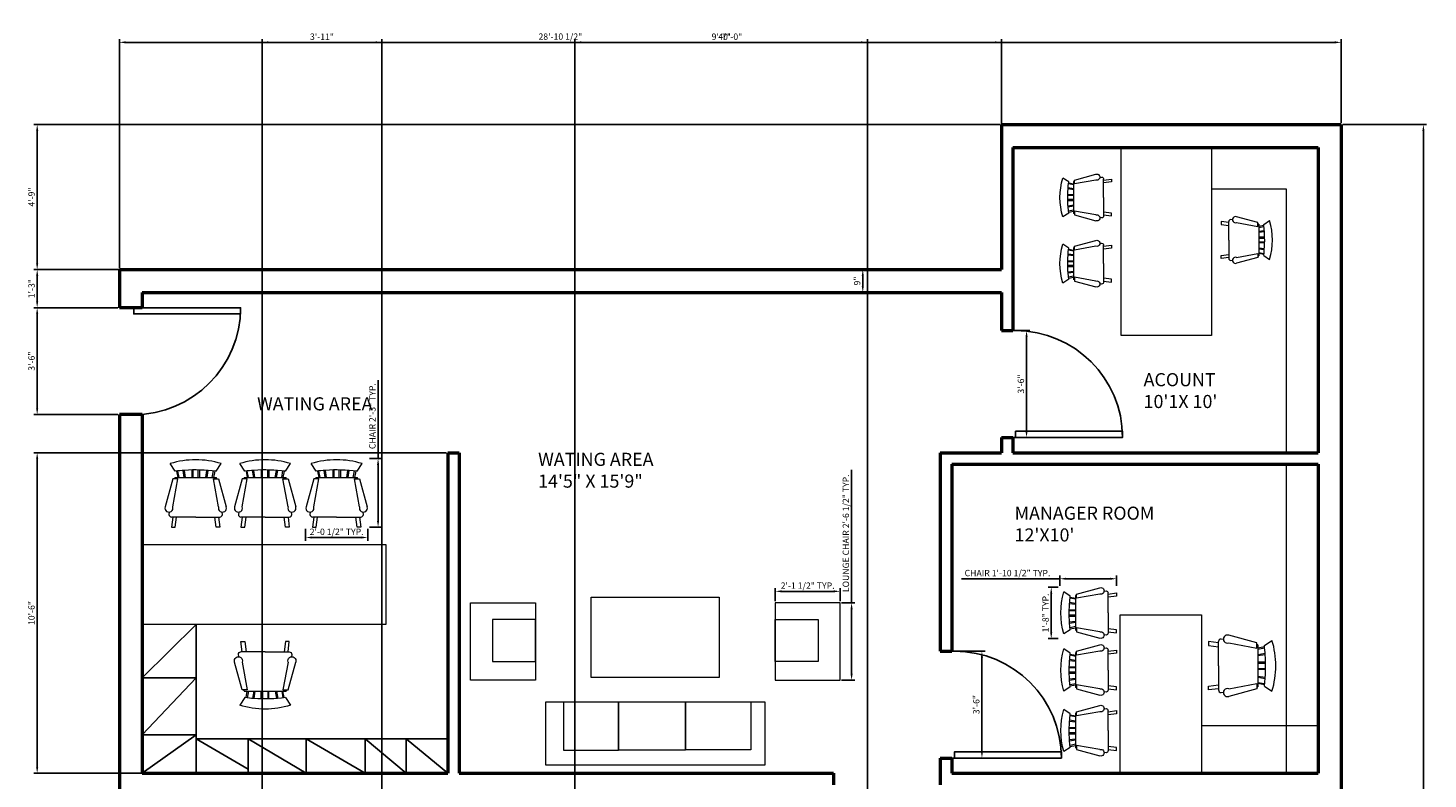
# Model space of a CAD drawing. Units: inches. Extents: x -4852 to -4300, y 4342 to 5059.
# Tile 4 of 4: x -4850 to -4300, y 4764 to 5059. Entities that reach past the tile are written whole.
import ezdxf

# ---------------------------------------------------------------- set-up
doc = ezdxf.new("R2010")
doc.units = ezdxf.units.IN
for name, color, linetype, lineweight in [('A-ANNO-DIMS', 2, 'Continuous', 18), ('A-AREA-IDEN', 7, 'Continuous', 18), ('A-DOOR', 4, 'Continuous', 25), ('A-FLOR-CASE', 9, 'Continuous', 25), ('A-FURN', 8, 'Continuous', 18), ('A-WALL', 7, 'Continuous', 50)]:
    doc.layers.add(name, color=color, linetype=linetype, lineweight=lineweight)
doc.styles.get("Standard").update_dxf_attribs({"font": 'arial.ttf'})
doc.dimstyles.new('ISO-25', dxfattribs={"dimtxt": 2.5, "dimasz": 2.5, "dimexe": 1.25, "dimexo": 0.625, "dimtad": 1, "dimdec": 0, "dimlunit": 3, "dimtxsty": 'Standard', "dimcen": 2.5, "dimadec": 0, "dimazin": 0, "dimtfac": 1, "dimtdec": 0, "dimtmove": 0, "dimatfit": 3, "dimfxl": 1, "dimarcsym": 0})

# ---------------------------------------------------------------- blocks, each defined once
blk = doc.blocks.new('*U2')
for p, q in [((0, 0), (0, -100)), ((750, 0), (750, -100))]:
    blk.add_line(p, q)
blk.add_lwpolyline([(0, 0), (0, 750), (43.75, 750), (43.75, 0)], close=True)
blk.add_arc((0, 0), 750, 0, 90)
blk = doc.blocks.new('Chair - Rocking')
for p, q in [((-8, -4.5), (-10, -1.5)), ((-7.5, -4.5), (-7, -7)), ((-6.5, -7), (-7.02225, -4.43)), ((-4.5, -7), (-4.96674, -4.19951)), ((-4, -7), (-4.40532, -4.16272)), ((-1.5, -4.05012), (-1.5, -7)), ((-1, -7), (-1, -4.05012)), ((1, -7), (1, -4.04655)), ((1.5, -4.05012), (1.5, -7)), ((4, -7), (4.40187, -4.18694)), ((4.5, -7), (4.96761, -4.19437)), ((6.5, -7), (7, -4.4057)), ((7.5, -4.5), (7, -7)), ((8, -4.5), (10, -1.5)), ((-9, -7.5), (-12, -18.49999)), ((-7, -7.5), (-9, -7.5)), ((-9, -18.49999), (-7, -7.5)), ((-8.23428, -6.99939), (-8.3093, -7.47958)), ((-8.23041, -7), (8.23915, -7)), ((7, -7.5), (9, -7.5)), ((9, -18.49999), (7, -7.5)), ((8.31071, -7.48854), (8.23449, -7.00073)), ((9, -7.5), (12, -18.49999)), ((-10.36644, -20.64523), (-10.5, -21.49999)), ((10.5, -21.49999), (10.3575, -20.58798)), ((-9, -22.49999), (-9.5, -26.49999)), ((0, -22.49999), (-9.5, -22.49999)), ((-9.5, -26.49999), (-8, -26.49999)), ((-8, -26.49999), (-7.5, -22.49999)), ((0, -22.49999), (9.5, -22.49999)), ((8, -26.49999), (7.5, -22.49999)), ((9.5, -26.49999), (8, -26.49999)), ((9, -22.49999), (9.5, -26.49999))]:
    blk.add_line(p, q)
for centre, radius, start, end in [((0, -34.08333), 34.08333, 72.93847, 107.0615), ((0, -68.25004), 64.25, 93.92211, 97.15267), ((0, -68.25004), 64.25, 82.84733, 93.92211), ((-10.5, -18.99999), 1.58114, 161.5651, 18.43495), ((-9.5, -21.49999), 1, 180, 270), ((10.5, -18.99999), 1.58114, 161.5651, 18.43495), ((9.5, -21.49999), 1, 270, 0)]:
    blk.add_arc(centre, radius, start, end)
blk = doc.blocks.new('*D7')
at = {"layer": 'A-ANNO-DIMS', "color": 0, "lineweight": -2, "transparency": 16777216}
for p, q in [((-4468.02, 4964.38), (-4523.09, 4964.38)), ((-4521.84, 4961.88), (-4521.84, 4957.88)), ((-4468.02, 4955.38), (-4523.09, 4955.38))]:
    blk.add_line(p, q, dxfattribs=at)
at = {"layer": 'A-ANNO-DIMS', "color": 0, "transparency": 16777216}
for points in [[(-4522.26, 4961.88), (-4521.43, 4961.88), (-4521.84, 4964.38)], [(-4522.26, 4957.88), (-4521.43, 4957.88), (-4521.84, 4955.38)]]:
    blk.add_solid(points, dxfattribs=at)
at = {"layer": 'Defpoints', "color": 0, "transparency": 16777216}
for p in [(-4467.4, 4964.38), (-4521.84, 4955.38), (-4467.4, 4955.38)]:
    blk.add_point(p, dxfattribs=at)
at = {"layer": 'A-ANNO-DIMS', "color": 0, "transparency": 16777216, "insert": (-4523.74, 4959.88), "char_height": 2.5, "attachment_point": 5, "rotation": 90}
blk.add_mtext('9"', dxfattribs=at)
blk = doc.blocks.new('*D14')
at = {"layer": 'A-ANNO-DIMS', "color": 0, "lineweight": -2, "transparency": 16777216}
for p, q in [((-4490.77, 4814.38), (-4473.78, 4814.38)), ((-4475.03, 4811.88), (-4475.03, 4774.88)), ((-4490.77, 4772.38), (-4473.78, 4772.38))]:
    blk.add_line(p, q, dxfattribs=at)
at = {"layer": 'A-ANNO-DIMS', "color": 0, "transparency": 16777216}
for points in [[(-4475.45, 4811.88), (-4474.62, 4811.88), (-4475.03, 4814.38)], [(-4475.45, 4774.88), (-4474.62, 4774.88), (-4475.03, 4772.38)]]:
    blk.add_solid(points, dxfattribs=at)
at = {"layer": 'Defpoints', "color": 0, "transparency": 16777216}
for p in [(-4491.4, 4814.38), (-4491.4, 4772.38), (-4475.03, 4772.38)]:
    blk.add_point(p, dxfattribs=at)
at = {"layer": 'A-ANNO-DIMS', "color": 0, "transparency": 16777216, "insert": (-4476.93, 4793.38), "char_height": 2.5, "attachment_point": 5, "rotation": 90}
blk.add_mtext('3\'-6"', dxfattribs=at)
blk = doc.blocks.new('*D15')
at = {"layer": 'A-ANNO-DIMS', "color": 0, "lineweight": -2, "transparency": 16777216}
for p, q in [((-4466.77, 4940.38), (-4456.25, 4940.38)), ((-4457.5, 4937.88), (-4457.5, 4900.88)), ((-4466.77, 4898.38), (-4456.25, 4898.38))]:
    blk.add_line(p, q, dxfattribs=at)
at = {"layer": 'A-ANNO-DIMS', "color": 0, "transparency": 16777216}
for points in [[(-4457.92, 4937.88), (-4457.08, 4937.88), (-4457.5, 4940.38)], [(-4457.92, 4900.88), (-4457.08, 4900.88), (-4457.5, 4898.38)]]:
    blk.add_solid(points, dxfattribs=at)
at = {"layer": 'Defpoints', "color": 0, "transparency": 16777216}
for p in [(-4467.4, 4940.38), (-4467.4, 4898.38), (-4457.5, 4898.38)]:
    blk.add_point(p, dxfattribs=at)
at = {"layer": 'A-ANNO-DIMS', "color": 0, "transparency": 16777216, "insert": (-4459.4, 4919.38), "char_height": 2.5, "attachment_point": 5, "rotation": 90}
blk.add_mtext('3\'-6"', dxfattribs=at)
blk = doc.blocks.new('CHAIR-LOUNGE')
for points in [[(0, 30.36), (25.44, 30.36), (25.44, 0), (0, 0)], [(25.44, 23.89), (8.61, 23.89), (8.61, 7.35), (25.44, 7.35)]]:
    blk.add_lwpolyline(points, close=True)
blk = doc.blocks.new('*D19')
at = {"layer": 'A-ANNO-DIMS', "color": 0, "lineweight": -2, "transparency": 16777216}
for p, q in [((-4712.28, 4890.11), (-4712.28, 4920.91)), ((-4715.71, 4890.11), (-4711.03, 4890.11)), ((-4712.28, 4865.61), (-4712.28, 4887.61)), ((-4715.71, 4863.11), (-4711.03, 4863.11))]:
    blk.add_line(p, q, dxfattribs=at)
at = {"layer": 'A-ANNO-DIMS', "color": 0, "transparency": 16777216}
for points in [[(-4712.7, 4887.61), (-4711.86, 4887.61), (-4712.28, 4890.11)], [(-4712.7, 4865.61), (-4711.86, 4865.61), (-4712.28, 4863.11)]]:
    blk.add_solid(points, dxfattribs=at)
at = {"layer": 'Defpoints', "color": 0, "transparency": 16777216}
for p in [(-4716.33, 4890.11), (-4712.28, 4890.11), (-4716.33, 4863.11)]:
    blk.add_point(p, dxfattribs=at)
at = {"layer": 'A-ANNO-DIMS', "color": 0, "transparency": 16777216, "insert": (-4714.2, 4906.76), "char_height": 2.5, "attachment_point": 5, "rotation": 90}
blk.add_mtext('CHAIR 2\'-3" TYP.', dxfattribs=at)
blk = doc.blocks.new('*D20')
at = {"layer": 'A-ANNO-DIMS', "color": 0, "lineweight": -2, "transparency": 16777216}
for p, q in [((-4740.77, 4862.49), (-4740.77, 4857.81)), ((-4716.33, 4862.49), (-4716.33, 4857.81)), ((-4738.27, 4859.06), (-4718.83, 4859.06))]:
    blk.add_line(p, q, dxfattribs=at)
at = {"layer": 'A-ANNO-DIMS', "color": 0, "transparency": 16777216}
for points in [[(-4738.27, 4859.48), (-4738.27, 4858.65), (-4740.77, 4859.06)], [(-4718.83, 4859.48), (-4718.83, 4858.65), (-4716.33, 4859.06)]]:
    blk.add_solid(points, dxfattribs=at)
at = {"layer": 'Defpoints', "color": 0, "transparency": 16777216}
for p in [(-4740.77, 4863.11), (-4716.33, 4863.11), (-4716.33, 4859.06)]:
    blk.add_point(p, dxfattribs=at)
at = {"layer": 'A-ANNO-DIMS', "color": 0, "transparency": 16777216, "insert": (-4728.55, 4860.98), "char_height": 2.5, "attachment_point": 5}
blk.add_mtext('2\'-0 1/2" TYP.', dxfattribs=at)
blk = doc.blocks.new('*D21')
at = {"layer": 'A-ANNO-DIMS', "color": 0, "lineweight": -2, "transparency": 16777216}
for p, q in [((-4444.45, 4842.85), (-4483.02, 4842.85)), ((-4444.45, 4840.12), (-4444.45, 4844.1)), ((-4424.64, 4842.85), (-4441.95, 4842.85)), ((-4422.14, 4840.12), (-4422.14, 4844.1))]:
    blk.add_line(p, q, dxfattribs=at)
at = {"layer": 'A-ANNO-DIMS', "color": 0, "transparency": 16777216}
for points in [[(-4441.95, 4843.26), (-4441.95, 4842.43), (-4444.45, 4842.85)], [(-4424.64, 4843.26), (-4424.64, 4842.43), (-4422.14, 4842.85)]]:
    blk.add_solid(points, dxfattribs=at)
at = {"layer": 'Defpoints', "color": 0, "transparency": 16777216}
for p in [(-4444.45, 4842.85), (-4444.45, 4839.5), (-4422.14, 4839.5)]:
    blk.add_point(p, dxfattribs=at)
at = {"layer": 'A-ANNO-DIMS', "color": 0, "transparency": 16777216, "insert": (-4464.99, 4844.76), "char_height": 2.5, "attachment_point": 5}
blk.add_mtext('CHAIR 1\'-10 1/2" TYP.', dxfattribs=at)
blk = doc.blocks.new('*D22')
at = {"layer": 'A-ANNO-DIMS', "color": 0, "lineweight": -2, "transparency": 16777216}
for p, q in [((-4445.08, 4839.5), (-4449.05, 4839.5)), ((-4447.8, 4837), (-4447.8, 4821.8)), ((-4445.08, 4819.3), (-4449.05, 4819.3))]:
    blk.add_line(p, q, dxfattribs=at)
at = {"layer": 'A-ANNO-DIMS', "color": 0, "transparency": 16777216}
for points in [[(-4448.22, 4837), (-4447.39, 4837), (-4447.8, 4839.5)], [(-4448.22, 4821.8), (-4447.39, 4821.8), (-4447.8, 4819.3)]]:
    blk.add_solid(points, dxfattribs=at)
at = {"layer": 'Defpoints', "color": 0, "transparency": 16777216}
for p in [(-4444.45, 4839.5), (-4447.8, 4819.3), (-4444.45, 4819.3)]:
    blk.add_point(p, dxfattribs=at)
at = {"layer": 'A-ANNO-DIMS', "color": 0, "transparency": 16777216, "insert": (-4449.7, 4829.4), "char_height": 2.5, "attachment_point": 5, "rotation": 90}
blk.add_mtext('1\'-8" TYP.', dxfattribs=at)
blk = doc.blocks.new('*D25')
at = {"layer": 'A-ANNO-DIMS', "color": 0, "lineweight": -2, "transparency": 16777216}
for p, q in [((-4526.24, 4833.34), (-4526.24, 4885.6)), ((-4530.17, 4833.34), (-4524.99, 4833.34)), ((-4526.24, 4805.48), (-4526.24, 4830.84)), ((-4530.17, 4802.98), (-4524.99, 4802.98))]:
    blk.add_line(p, q, dxfattribs=at)
at = {"layer": 'A-ANNO-DIMS', "color": 0, "transparency": 16777216}
for points in [[(-4526.66, 4830.84), (-4525.82, 4830.84), (-4526.24, 4833.34)], [(-4526.66, 4805.48), (-4525.82, 4805.48), (-4526.24, 4802.98)]]:
    blk.add_solid(points, dxfattribs=at)
at = {"layer": 'Defpoints', "color": 0, "transparency": 16777216}
for p in [(-4530.79, 4833.34), (-4526.24, 4833.34), (-4530.79, 4802.98)]:
    blk.add_point(p, dxfattribs=at)
at = {"layer": 'A-ANNO-DIMS', "color": 0, "transparency": 16777216, "insert": (-4528.16, 4860.72), "char_height": 2.5, "attachment_point": 5, "rotation": 90}
blk.add_mtext('LOUNGE CHAIR 2\'-6 1/2" TYP.', dxfattribs=at)
blk = doc.blocks.new('*D26')
at = {"layer": 'A-ANNO-DIMS', "color": 0, "lineweight": -2, "transparency": 16777216}
for p, q in [((-4556.23, 4833.97), (-4556.23, 4839.15)), ((-4533.29, 4837.9), (-4553.73, 4837.9)), ((-4530.79, 4833.97), (-4530.79, 4839.15))]:
    blk.add_line(p, q, dxfattribs=at)
at = {"layer": 'A-ANNO-DIMS', "color": 0, "transparency": 16777216}
for points in [[(-4553.73, 4838.31), (-4553.73, 4837.48), (-4556.23, 4837.9)], [(-4533.29, 4838.31), (-4533.29, 4837.48), (-4530.79, 4837.9)]]:
    blk.add_solid(points, dxfattribs=at)
at = {"layer": 'Defpoints', "color": 0, "transparency": 16777216}
for p in [(-4556.23, 4837.9), (-4556.23, 4833.34), (-4530.79, 4833.34)]:
    blk.add_point(p, dxfattribs=at)
at = {"layer": 'A-ANNO-DIMS', "color": 0, "transparency": 16777216, "insert": (-4543.51, 4839.81), "char_height": 2.5, "attachment_point": 5}
blk.add_mtext('2\'-1 1/2" TYP.', dxfattribs=at)
blk = doc.blocks.new('*D39')
at = {"layer": 'A-ANNO-DIMS', "color": 0, "lineweight": -2, "transparency": 16777216}
for p, q in [((-4813.9, 4965), (-4813.9, 5054.94)), ((-4333.9, 5022), (-4333.9, 5054.94)), ((-4811.4, 5053.69), (-4336.4, 5053.69))]:
    blk.add_line(p, q, dxfattribs=at)
at = {"layer": 'A-ANNO-DIMS', "color": 0, "transparency": 16777216}
for points in [[(-4811.4, 5054.11), (-4811.4, 5053.27), (-4813.9, 5053.69)], [(-4336.4, 5054.11), (-4336.4, 5053.27), (-4333.9, 5053.69)]]:
    blk.add_solid(points, dxfattribs=at)
at = {"layer": 'Defpoints', "color": 0, "transparency": 16777216}
for p in [(-4333.9, 5053.69), (-4333.9, 5021.38), (-4813.9, 4964.38)]:
    blk.add_point(p, dxfattribs=at)
at = {"layer": 'A-ANNO-DIMS', "color": 0, "transparency": 16777216, "insert": (-4573.9, 5055.59), "char_height": 2.5, "attachment_point": 5}
blk.add_mtext('40\'-0"', dxfattribs=at)
blk = doc.blocks.new('*D40')
at = {"layer": 'A-ANNO-DIMS', "color": 0, "lineweight": -2, "transparency": 16777216}
for p, q in [((-4333.27, 5021.38), (-4300.34, 5021.38)), ((-4301.59, 4422.38), (-4301.59, 5018.88)), ((-4333.27, 4419.88), (-4300.34, 4419.88))]:
    blk.add_line(p, q, dxfattribs=at)
at = {"layer": 'A-ANNO-DIMS', "color": 0, "transparency": 16777216}
for points in [[(-4302.01, 5018.88), (-4301.17, 5018.88), (-4301.59, 5021.38)], [(-4302.01, 4422.38), (-4301.17, 4422.38), (-4301.59, 4419.88)]]:
    blk.add_solid(points, dxfattribs=at)
at = {"layer": 'Defpoints', "color": 0, "transparency": 16777216}
for p in [(-4333.9, 5021.38), (-4301.59, 5021.38), (-4333.9, 4419.88)]:
    blk.add_point(p, dxfattribs=at)
at = {"layer": 'A-ANNO-DIMS', "color": 0, "transparency": 16777216, "insert": (-4303.51, 4720.63), "char_height": 2.5, "attachment_point": 5, "rotation": 90}
blk.add_mtext('50\'-1 1/2"', dxfattribs=at)
blk = doc.blocks.new('*D41')
at = {"layer": 'A-ANNO-DIMS', "color": 0, "lineweight": -2, "transparency": 16777216}
for p, q in [((-4813.9, 4965), (-4813.9, 5054.94)), ((-4467.4, 4965), (-4467.4, 5054.94)), ((-4811.4, 5053.69), (-4469.9, 5053.69))]:
    blk.add_line(p, q, dxfattribs=at)
at = {"layer": 'A-ANNO-DIMS', "color": 0, "transparency": 16777216}
for points in [[(-4811.4, 5054.11), (-4811.4, 5053.27), (-4813.9, 5053.69)], [(-4469.9, 5054.11), (-4469.9, 5053.27), (-4467.4, 5053.69)]]:
    blk.add_solid(points, dxfattribs=at)
at = {"layer": 'Defpoints', "color": 0, "transparency": 16777216}
for p in [(-4467.4, 5053.69), (-4813.9, 4964.38), (-4467.4, 4964.38)]:
    blk.add_point(p, dxfattribs=at)
at = {"layer": 'A-ANNO-DIMS', "color": 0, "transparency": 16777216, "insert": (-4640.65, 5055.61), "char_height": 2.5, "attachment_point": 5}
blk.add_mtext('28\'-10 1/2"', dxfattribs=at)
blk = doc.blocks.new('*D42')
at = {"layer": 'A-ANNO-DIMS', "color": 0, "lineweight": -2, "transparency": 16777216}
for p, q in [((-4468.02, 5021.38), (-4847.46, 5021.38)), ((-4846.21, 4966.88), (-4846.21, 5018.88)), ((-4468.02, 4964.38), (-4847.46, 4964.38))]:
    blk.add_line(p, q, dxfattribs=at)
at = {"layer": 'A-ANNO-DIMS', "color": 0, "transparency": 16777216}
for points in [[(-4846.63, 5018.88), (-4845.79, 5018.88), (-4846.21, 5021.38)], [(-4846.63, 4966.88), (-4845.79, 4966.88), (-4846.21, 4964.38)]]:
    blk.add_solid(points, dxfattribs=at)
at = {"layer": 'Defpoints', "color": 0, "transparency": 16777216}
for p in [(-4846.21, 5021.38), (-4467.4, 5021.38), (-4467.4, 4964.38)]:
    blk.add_point(p, dxfattribs=at)
at = {"layer": 'A-ANNO-DIMS', "color": 0, "transparency": 16777216, "insert": (-4848.11, 4992.88), "char_height": 2.5, "attachment_point": 5, "rotation": 90}
blk.add_mtext('4\'-9"', dxfattribs=at)
blk = doc.blocks.new('*D45')
at = {"layer": 'A-ANNO-DIMS', "color": 0, "lineweight": -2, "transparency": 16777216}
for p, q in [((-4814.52, 4949.38), (-4847.46, 4949.38)), ((-4846.21, 4909.88), (-4846.21, 4946.88)), ((-4814.52, 4907.38), (-4847.46, 4907.38))]:
    blk.add_line(p, q, dxfattribs=at)
at = {"layer": 'A-ANNO-DIMS', "color": 0, "transparency": 16777216}
for points in [[(-4846.63, 4946.88), (-4845.79, 4946.88), (-4846.21, 4949.38)], [(-4846.63, 4909.88), (-4845.79, 4909.88), (-4846.21, 4907.38)]]:
    blk.add_solid(points, dxfattribs=at)
at = {"layer": 'Defpoints', "color": 0, "transparency": 16777216}
for p in [(-4846.21, 4949.38), (-4813.9, 4949.38), (-4813.9, 4907.38)]:
    blk.add_point(p, dxfattribs=at)
at = {"layer": 'A-ANNO-DIMS', "color": 0, "transparency": 16777216, "insert": (-4848.11, 4928.38), "char_height": 2.5, "attachment_point": 5, "rotation": 90}
blk.add_mtext('3\'-6"', dxfattribs=at)
blk = doc.blocks.new('*D49')
at = {"layer": 'A-ANNO-DIMS', "color": 0, "lineweight": -2, "transparency": 16777216}
for p, q in [((-4814.52, 4964.38), (-4847.46, 4964.38)), ((-4846.21, 4951.88), (-4846.21, 4961.88)), ((-4814.52, 4949.38), (-4847.46, 4949.38))]:
    blk.add_line(p, q, dxfattribs=at)
at = {"layer": 'A-ANNO-DIMS', "color": 0, "transparency": 16777216}
for points in [[(-4846.63, 4961.88), (-4845.79, 4961.88), (-4846.21, 4964.38)], [(-4846.63, 4951.88), (-4845.79, 4951.88), (-4846.21, 4949.38)]]:
    blk.add_solid(points, dxfattribs=at)
at = {"layer": 'Defpoints', "color": 0, "transparency": 16777216}
for p in [(-4846.21, 4964.38), (-4813.9, 4964.38), (-4813.9, 4949.38)]:
    blk.add_point(p, dxfattribs=at)
at = {"layer": 'A-ANNO-DIMS', "color": 0, "transparency": 16777216, "insert": (-4848.11, 4956.88), "char_height": 2.5, "attachment_point": 5, "rotation": 90}
blk.add_mtext('1\'-3"', dxfattribs=at)
blk = doc.blocks.new('*D58')
at = {"layer": 'A-ANNO-DIMS', "color": 0, "lineweight": -2, "transparency": 16777216}
for p, q in [((-4685.52, 4892.38), (-4847.46, 4892.38)), ((-4846.21, 4768.88), (-4846.21, 4889.88)), ((-4685.52, 4766.38), (-4847.46, 4766.38))]:
    blk.add_line(p, q, dxfattribs=at)
at = {"layer": 'A-ANNO-DIMS', "color": 0, "transparency": 16777216}
for points in [[(-4846.63, 4889.88), (-4845.79, 4889.88), (-4846.21, 4892.38)], [(-4846.63, 4768.88), (-4845.79, 4768.88), (-4846.21, 4766.38)]]:
    blk.add_solid(points, dxfattribs=at)
at = {"layer": 'Defpoints', "color": 0, "transparency": 16777216}
for p in [(-4846.21, 4892.38), (-4684.9, 4892.38), (-4684.9, 4766.38)]:
    blk.add_point(p, dxfattribs=at)
at = {"layer": 'A-ANNO-DIMS', "color": 0, "transparency": 16777216, "insert": (-4848.11, 4829.38), "char_height": 2.5, "attachment_point": 5, "rotation": 90}
blk.add_mtext('10\'-6"', dxfattribs=at)
blk = doc.blocks.new('*D60')
at = {"layer": 'A-ANNO-DIMS', "color": 0, "lineweight": -2, "transparency": 16777216}
for p, q in [((-4634.93, 4696.96), (-4634.93, 5054.94)), ((-4519.98, 4696.96), (-4519.98, 5054.94)), ((-4632.43, 5053.69), (-4522.48, 5053.69))]:
    blk.add_line(p, q, dxfattribs=at)
at = {"layer": 'A-ANNO-DIMS', "color": 0, "transparency": 16777216}
for points in [[(-4632.43, 5054.11), (-4632.43, 5053.27), (-4634.93, 5053.69)], [(-4522.48, 5054.11), (-4522.48, 5053.27), (-4519.98, 5053.69)]]:
    blk.add_solid(points, dxfattribs=at)
at = {"layer": 'Defpoints', "color": 0, "transparency": 16777216}
for p in [(-4519.98, 5053.69), (-4634.93, 4696.34), (-4519.98, 4696.34)]:
    blk.add_point(p, dxfattribs=at)
at = {"layer": 'A-ANNO-DIMS', "color": 0, "transparency": 16777216, "insert": (-4577.45, 5055.59), "char_height": 2.5, "attachment_point": 5}
blk.add_mtext('9\'-7"', dxfattribs=at)
blk = doc.blocks.new('*D62')
at = {"layer": 'A-ANNO-DIMS', "color": 0, "lineweight": -2, "transparency": 16777216}
for p, q in [((-4757.87, 4455.31), (-4757.87, 5054.94)), ((-4710.76, 4455.31), (-4710.76, 5054.94)), ((-4755.37, 5053.69), (-4713.26, 5053.69))]:
    blk.add_line(p, q, dxfattribs=at)
at = {"layer": 'A-ANNO-DIMS', "color": 0, "transparency": 16777216}
for points in [[(-4755.37, 5054.11), (-4755.37, 5053.27), (-4757.87, 5053.69)], [(-4713.26, 5054.11), (-4713.26, 5053.27), (-4710.76, 5053.69)]]:
    blk.add_solid(points, dxfattribs=at)
at = {"layer": 'Defpoints', "color": 0, "transparency": 16777216}
for p in [(-4710.76, 5053.69), (-4757.87, 4454.69), (-4710.76, 4454.69)]:
    blk.add_point(p, dxfattribs=at)
at = {"layer": 'A-ANNO-DIMS', "color": 0, "transparency": 16777216, "insert": (-4734.32, 5055.59), "char_height": 2.5, "attachment_point": 5}
blk.add_mtext('3\'-11"', dxfattribs=at)

msp = doc.modelspace()

# ---------------------------------------------------------------- linework, layer by layer
at = {"layer": 'A-FLOR-CASE'}
for p, q in [((-4783.75, 4824.92), (-4804.9, 4803.94)), ((-4783.75, 4824.92), (-4783.75, 4779.95)), ((-4804.9, 4803.94), (-4783.75, 4803.94)), ((-4783.75, 4803.94), (-4804.9, 4781.54)), ((-4804.9, 4781.54), (-4783.75, 4781.54)), ((-4783.75, 4781.54), (-4804.9, 4766.38)), ((-4783.75, 4779.95), (-4684.9, 4779.95)), ((-4783.75, 4779.95), (-4783.75, 4766.38)), ((-4783.75, 4779.95), (-4763.33, 4768.03)), ((-4763.33, 4779.95), (-4763.33, 4766.38)), ((-4763.33, 4779.95), (-4740.53, 4766.38)), ((-4740.53, 4779.95), (-4740.53, 4766.38)), ((-4740.53, 4779.95), (-4717.34, 4766.38)), ((-4717.34, 4779.95), (-4717.34, 4766.38)), ((-4717.34, 4779.95), (-4701.27, 4766.38)), ((-4701.27, 4779.95), (-4701.27, 4766.38)), ((-4701.27, 4779.95), (-4684.9, 4766.38))]:
    msp.add_line(p, q, dxfattribs=at)
at = {"layer": 'A-FURN'}
for p, q in [((-4355.43, 4995.96), (-4384.9, 4995.96)), ((-4355.43, 4892.38), (-4355.43, 4995.96)), ((-4355.43, 4766.38), (-4355.43, 4887.88)), ((-4388.82, 4785.11), (-4342.9, 4785.11))]:
    msp.add_line(p, q, dxfattribs=at)
for points in [[(-4420.38, 5012.38), (-4384.9, 5012.38), (-4384.9, 4938.44), (-4420.38, 4938.44)], [(-4804.9, 4856.31), (-4709.21, 4856.31), (-4709.21, 4824.92), (-4804.9, 4824.92)], [(-4628.62, 4835.61), (-4578.32, 4835.61), (-4578.32, 4804.05), (-4628.62, 4804.05)], [(-4420.71, 4828.71), (-4388.82, 4828.71), (-4388.82, 4766.38), (-4420.71, 4766.38)], [(-4646.34, 4794.45), (-4560.36, 4794.45), (-4560.36, 4769.6), (-4646.34, 4769.6)], [(-4639.26, 4794.45), (-4617.86, 4794.45), (-4617.86, 4775.28), (-4639.26, 4775.28)], [(-4617.86, 4794.45), (-4591.53, 4794.45), (-4591.53, 4775.45), (-4617.86, 4775.45)], [(-4591.53, 4794.45), (-4565.86, 4794.45), (-4565.86, 4775.61), (-4591.53, 4775.61)]]:
    msp.add_lwpolyline(points, close=True, dxfattribs=at)
at = {"layer": 'A-WALL'}
for p, q in [((-4467.4, 5021.38), (-4333.9, 5021.38)), ((-4467.4, 5021.38), (-4467.4, 4964.38)), ((-4333.9, 5021.38), (-4333.9, 4706.38)), ((-4462.9, 5012.38), (-4342.9, 5012.38)), ((-4462.9, 5012.38), (-4462.9, 4940.38)), ((-4342.9, 5012.38), (-4342.9, 4892.38)), ((-4813.9, 4964.38), (-4813.9, 4949.38)), ((-4813.9, 4964.38), (-4467.4, 4964.38)), ((-4804.9, 4955.38), (-4804.9, 4949.38)), ((-4804.9, 4955.38), (-4467.4, 4955.38)), ((-4467.4, 4955.38), (-4467.4, 4940.38)), ((-4804.9, 4949.38), (-4813.9, 4949.38)), ((-4467.4, 4940.38), (-4462.9, 4940.38)), ((-4804.9, 4907.38), (-4813.9, 4907.38)), ((-4813.9, 4907.38), (-4813.9, 4419.88)), ((-4804.9, 4907.38), (-4804.9, 4766.38)), ((-4467.4, 4898.38), (-4462.9, 4898.38)), ((-4467.4, 4898.38), (-4467.4, 4892.38)), ((-4462.9, 4898.38), (-4462.9, 4892.38)), ((-4684.9, 4892.38), (-4680.4, 4892.38)), ((-4684.9, 4892.38), (-4684.9, 4766.38)), ((-4680.4, 4892.38), (-4680.4, 4766.38)), ((-4491.4, 4892.38), (-4467.4, 4892.38)), ((-4491.4, 4892.38), (-4491.4, 4814.38)), ((-4491.4, 4892.38), (-4467.4, 4892.38)), ((-4462.9, 4892.38), (-4342.9, 4892.38)), ((-4486.9, 4887.88), (-4486.9, 4814.38)), ((-4486.9, 4887.88), (-4342.9, 4887.88)), ((-4342.9, 4887.88), (-4342.9, 4766.38)), ((-4491.4, 4814.38), (-4486.9, 4814.38)), ((-4491.4, 4772.38), (-4486.9, 4772.38)), ((-4491.4, 4772.38), (-4491.4, 4761.88)), ((-4486.9, 4772.38), (-4486.9, 4766.38)), ((-4804.9, 4766.38), (-4684.9, 4766.38)), ((-4680.4, 4766.38), (-4533.4, 4766.38)), ((-4664.4, 4766.38), (-4533.4, 4766.38)), ((-4533.4, 4766.38), (-4533.4, 4761.88)), ((-4486.9, 4766.38), (-4342.9, 4766.38))]:
    msp.add_line(p, q, dxfattribs=at)

# ---------------------------------------------------------------- block references
at = {"layer": 'A-DOOR', "yscale": 0.0559999999999998, "zscale": 0.0559999999999998, "rotation": 270}
for p, xscale in [((-4808.3, 4949.38), 0.0559999999999998), ((-4461.8, 4898.38), -0.0559999999999998), ((-4485.8, 4772.38), -0.0559999999999998)]:
    msp.add_blockref('*U2', p, dxfattribs=dict(at, xscale=xscale))
at = {"layer": 'A-FURN'}
for p, xscale, yscale, zscale, rotation in [((-4444.38, 4992.7), -0.7621443616854127, 0.7621443616854127, 0.7621443616854127, 90), ((-4360.9, 4975.99), 0.7621443616854127, 0.7621443616854127, 0.7621443616854127, 270), ((-4444.38, 4966.7), -0.7621443616854127, 0.7621443616854127, 0.7621443616854127, 90), ((-4444.04, 4829.4), -0.8265392436159728, 0.8265392436159728, 0.8265392436159728, 90), ((-4444.04, 4806.97), -0.8265392436159728, 0.8265392436159728, 0.8265392436159728, 90), ((-4444.04, 4783.15), -0.8265392436159728, 0.8265392436159728, 0.8265392436159728, 90)]:
    msp.add_blockref('Chair - Rocking', p, dxfattribs=dict(at, xscale=xscale, yscale=yscale, zscale=zscale, rotation=rotation))
for name, p in [('Chair - Rocking', (-4783.94, 4889.61)), ('Chair - Rocking', (-4756.65, 4889.61)), ('Chair - Rocking', (-4728.55, 4889.61)), ('CHAIR-LOUNGE', (-4675.9, 4802.98))]:
    msp.add_blockref(name, p, dxfattribs=at)
at = {"layer": 'A-FURN', "extrusion": (0, 0, -1), "zscale": -1}
msp.add_blockref('CHAIR-LOUNGE', (4530.79, 4802.98), dxfattribs=at)
at = {"layer": 'A-FURN', "rotation": 270}
msp.add_blockref('Chair - Rocking', (-4359.57, 4808.62), dxfattribs=at)
at = {"layer": 'A-FURN', "xscale": -1, "rotation": 180}
msp.add_blockref('Chair - Rocking', (-4756.65, 4791.62), dxfattribs=at)

# ---------------------------------------------------------------- texts
at = {"layer": 'A-AREA-IDEN'}
for s, height, p in [('ACOUNT', 5.149, (-4411.52, 4918.52)), ('WATING AREA', 5.1489, (-4759.82, 4909.03)), ("10'1X 10'", 5.149, (-4411.52, 4909.95)), ('WATING AREA', 5.1489, (-4649.4, 4887.21)), ('14\'5" X 15\'9"', 5.1489, (-4649.4, 4878.65)), ('MANAGER ROOM ', 5.1489, (-4462.21, 4866.05)), ("12'X10'", 5.149, (-4462.21, 4857.49))]:
    msp.add_text(s, height=height, dxfattribs=at).set_placement(p)

# ---------------------------------------------------------------- dimensions: what is measured, and where the dimension line sits
at = {"layer": 'A-ANNO-DIMS'}
for base, p1, p2, picture, middle in [((-4467.4, 5053.69), (-4813.9, 4964.38), (-4467.4, 4964.38), '*D41', (-4640.65, 5055.61)), ((-4333.9, 5053.69), (-4813.9, 4964.38), (-4333.9, 5021.38), '*D39', (-4573.9, 5055.59)), ((-4710.76, 5053.69), (-4757.87, 4454.69), (-4710.76, 4454.69), '*D62', (-4734.32, 5055.59)), ((-4519.9791, 5053.6893), (-4634.9301, 4696.3372), (-4519.9791, 4696.3372), '*D60', (-4577.4546, 5055.5907))]:
    dim = msp.add_linear_dim(base=base, p1=p1, p2=p2, dimstyle='ISO-25', override={"dimdec": 1, "dimlfac": 1, "dimrnd": 0, "dimzin": 1, "dimdsep": 46, "dimlunit": 4, "dimfrac": 2}, dxfattribs=at)
    dim.commit()
    dim.dimension.update_dxf_attribs({"geometry": picture, "text_midpoint": middle})
for base, p1, p2, override, picture, middle in [((-4846.21, 5021.38), (-4467.4, 4964.38), (-4467.4, 5021.38), {"dimdec": 1, "dimlfac": 1, "dimrnd": 0, "dimzin": 1, "dimdsep": 46, "dimlunit": 4, "dimfrac": 2}, '*D42', (-4848.11, 4992.88)), ((-4301.59, 5021.38), (-4333.9, 4419.88), (-4333.9, 5021.38), {"dimdec": 1, "dimlfac": 1, "dimrnd": 0, "dimzin": 1, "dimdsep": 46, "dimlunit": 4, "dimfrac": 2}, '*D40', (-4303.51, 4720.63)), ((-4846.21, 4964.38), (-4813.9, 4949.38), (-4813.9, 4964.38), {"dimdec": 1, "dimlfac": 1, "dimrnd": 0, "dimzin": 1, "dimdsep": 46, "dimlunit": 4, "dimfrac": 2}, '*D49', (-4848.11, 4956.88)), ((-4521.84, 4955.38), (-4467.4, 4964.38), (-4467.4, 4955.38), {"dimclrd": 0, "dimclre": 0, "dimclrt": 0}, '*D7', (-4523.74, 4959.88)), ((-4846.21, 4949.38), (-4813.9, 4907.38), (-4813.9, 4949.38), {"dimdec": 1, "dimlfac": 1, "dimrnd": 0, "dimzin": 1, "dimdsep": 46, "dimlunit": 4, "dimfrac": 2}, '*D45', (-4848.11, 4928.38)), ((-4457.5, 4898.38), (-4467.4, 4940.38), (-4467.4, 4898.38), {"dimclrd": 0, "dimclre": 0, "dimclrt": 0}, '*D15', (-4459.4, 4919.38)), ((-4846.21, 4892.38), (-4684.9, 4766.38), (-4684.9, 4892.38), {"dimdec": 1, "dimlfac": 1, "dimrnd": 0, "dimzin": 1, "dimdsep": 46, "dimlunit": 4, "dimfrac": 2}, '*D58', (-4848.11, 4829.38)), ((-4475.03, 4772.38), (-4491.4, 4814.38), (-4491.4, 4772.38), {"dimclrd": 0, "dimclre": 0, "dimclrt": 0}, '*D14', (-4476.93, 4793.38))]:
    dim = msp.add_linear_dim(base=base, p1=p1, p2=p2, angle=90, dimstyle='ISO-25', override=override, dxfattribs=at)
    dim.commit()
    dim.dimension.update_dxf_attribs({"geometry": picture, "text_midpoint": middle})
for base, p1, p2, angle, text, picture, middle in [((-4712.28, 4890.11), (-4716.33, 4863.11), (-4716.33, 4890.11), 90, 'CHAIR <> TYP.', '*D19', (-4714.2, 4906.76)), ((-4526.24, 4833.34), (-4530.79, 4802.98), (-4530.79, 4833.34), 90, 'LOUNGE CHAIR <> TYP.', '*D25', (-4528.16, 4860.72)), ((-4444.45, 4842.85), (-4422.14, 4839.5), (-4444.45, 4839.5), 180, 'CHAIR <> TYP.', '*D21', (-4464.99, 4844.76)), ((-4556.23, 4837.9), (-4530.79, 4833.34), (-4556.23, 4833.34), 180, '<> TYP.', '*D26', (-4543.51, 4839.81)), ((-4447.8, 4819.3), (-4444.45, 4839.5), (-4444.45, 4819.3), 270, '<> TYP.', '*D22', (-4449.7, 4829.4))]:
    dim = msp.add_linear_dim(base=base, p1=p1, p2=p2, angle=angle, text=text, dimstyle='ISO-25', override={"dimdec": 1, "dimlfac": 1, "dimrnd": 0, "dimzin": 1, "dimdsep": 46, "dimlunit": 4, "dimfrac": 2}, dxfattribs=at)
    dim.commit()
    dim.dimension.update_dxf_attribs({"geometry": picture, "text_midpoint": middle})
dim = msp.add_linear_dim(base=(-4716.33, 4859.06), p1=(-4740.77, 4863.11), p2=(-4716.33, 4863.11), text='<> TYP.', dimstyle='ISO-25', override={"dimdec": 1, "dimlfac": 1, "dimrnd": 0, "dimzin": 1, "dimdsep": 46, "dimlunit": 4, "dimfrac": 2}, dxfattribs=at)
dim.commit()
dim.dimension.update_dxf_attribs({"geometry": '*D20', "text_midpoint": (-4728.55, 4860.98)})

doc.saveas('drawing.dxf')
